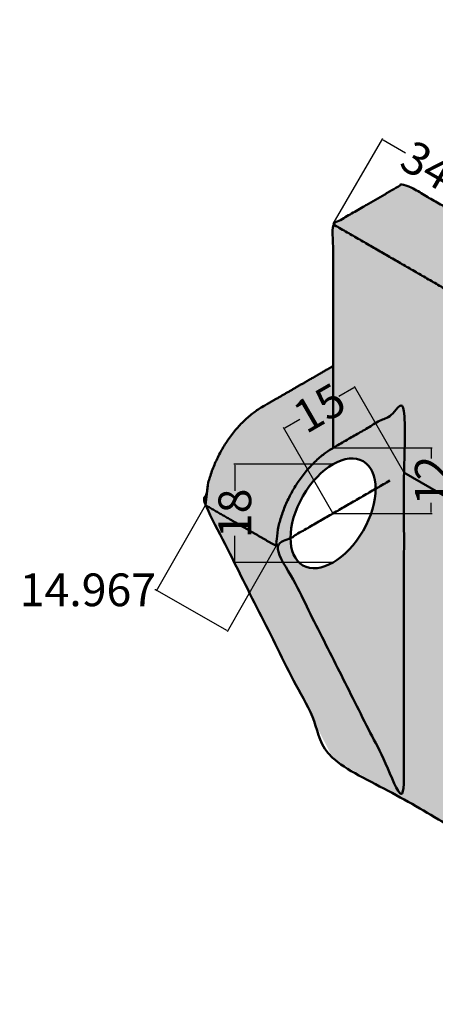
# Model space of a CAD drawing. Units: millimetres. Extents: x -57 to 165, y 2 to 198.
# Tile 1 of 1: x -57.4 to 18.8, y 17.5 to 198. Entities that reach past the tile are written whole.
import ezdxf

# ---------------------------------------------------------------- set-up
doc = ezdxf.new("R2010")
doc.units = ezdxf.units.MM
doc.header["$MEASUREMENT"] = 0
for name, color, linetype, lineweight in [('M-DIMS', 2, 'Continuous', 18), ('M-HATC', 8, 'Continuous', 18), ('M-OUTL', 7, 'Continuous', 50)]:
    doc.layers.add(name, color=color, linetype=linetype, lineweight=lineweight)
doc.styles.get("Standard").update_dxf_attribs({"font": 'arial.ttf'})
doc.dimstyles.get("Standard").update_dxf_attribs({"dimtxt": 6, "dimasz": 0.18, "dimexe": 0.18, "dimexo": 0.0625, "dimgap": 0.09, "dimtad": 0, "dimtoh": 1, "dimdec": 0, "dimzin": 0, "dimdsep": 46, "dimtxsty": 'Standard', "dimcen": 0.09, "dimadec": 0, "dimazin": 0, "dimtfac": 1, "dimtdec": 0, "dimtofl": 0, "dimtmove": 0, "dimatfit": 3, "dimfxl": 1, "dimtolj": 1, "dimtzin": 0, "dimarcsym": 0})

# ---------------------------------------------------------------- blocks, each defined once
blk = doc.blocks.new('*D13')
at = {"layer": 'Defpoints', "color": 0, "transparency": 16777216}
for p in [(-17.95371300000001, 116.497997), (0.046287, 116.497997), (0.046287, 98.49799700000005)]:
    blk.add_point(p, dxfattribs=at)
at = {"layer": 'M-DIMS', "color": 0, "lineweight": -2, "transparency": 16777216}
for p, q in [((-0.016213, 116.497997), (-18.13371300000001, 116.497997)), ((-17.95371300000001, 116.317997), (-17.95371300000001, 111.6091429754434)), ((-17.95371300000001, 98.67799700000006), (-17.95371300000001, 103.3868510245566)), ((-0.016213, 98.49799700000005), (-18.13371300000001, 98.49799700000005))]:
    blk.add_line(p, q, dxfattribs=at)
at = {"layer": 'M-DIMS', "color": 0, "transparency": 16777216}
for points in [[(-17.98371300000001, 116.317997), (-17.92371300000001, 116.317997), (-17.95371300000001, 116.497997)], [(-17.98371300000001, 98.67799700000006), (-17.92371300000001, 98.67799700000006), (-17.95371300000001, 98.49799700000005)]]:
    blk.add_solid(points, dxfattribs=at)
at = {"layer": 'M-DIMS', "color": 0, "transparency": 16777216, "insert": (-17.95371299999998, 107.497997), "char_height": 6, "attachment_point": 5, "rotation": 90}
blk.add_mtext('\\A1;18', dxfattribs=at)
blk = doc.blocks.new('*D17')
at = {"layer": 'Defpoints', "color": 0, "transparency": 16777216}
for p in [(0.0462869999999924, 160.497997), (39.30844832468702, 158.6118924312673), (30.307407, 143.024036)]:
    blk.add_point(p, dxfattribs=at)
at = {"layer": 'M-DIMS', "color": 0, "lineweight": -2, "transparency": 16777216}
for p, q in [((0.0775406150812756, 160.5521215004074), (9.137338633268897, 176.2417318143229)), ((9.203206783008142, 175.9958428417155), (13.32703206028853, 173.6145839495605)), ((39.1525697635137, 158.7019028427014), (35.0287444862333, 161.0831617348563)), ((30.33866061508128, 143.0781605004074), (39.39845873612112, 158.7677709924407))]:
    blk.add_line(p, q, dxfattribs=at)
at = {"layer": 'M-DIMS', "color": 0, "transparency": 16777216}
for points in [[(9.218208518247167, 176.021822601911), (9.18820504776913, 175.9698630815199), (9.047328221834803, 176.0858532531495)], [(39.16757149875272, 158.727882602897), (39.13756802827469, 158.6759230825059), (39.30844832468702, 158.6118924312673)]]:
    blk.add_solid(points, dxfattribs=at)
at = {"layer": 'M-DIMS', "color": 0, "transparency": 16777216, "insert": (24.17788827326091, 167.3488728422084), "char_height": 6, "attachment_point": 5, "rotation": 329.9961731765761}
blk.add_mtext('\\A1;34.944', dxfattribs=at)
blk = doc.blocks.new('*D19')
at = {"layer": 'Defpoints', "color": 0, "transparency": 16777216}
for p in [(0.046287, 119.497997), (0.046287, 107.497997), (18.04628700000001, 107.497997)]:
    blk.add_point(p, dxfattribs=at)
at = {"layer": 'M-DIMS', "color": 0, "lineweight": -2, "transparency": 16777216}
for p, q in [((0.108787, 119.497997), (18.22628700000001, 119.497997)), ((18.04628700000001, 119.317997), (18.04628700000001, 117.5723080504775)), ((18.04628700000001, 107.677997), (18.04628700000001, 109.4236859495225)), ((0.108787, 107.497997), (18.22628700000001, 107.497997))]:
    blk.add_line(p, q, dxfattribs=at)
at = {"layer": 'M-DIMS', "color": 0, "transparency": 16777216}
for points in [[(18.01628700000001, 119.317997), (18.07628700000001, 119.317997), (18.04628700000001, 119.497997)], [(18.01628700000001, 107.677997), (18.07628700000001, 107.677997), (18.04628700000001, 107.497997)]]:
    blk.add_solid(points, dxfattribs=at)
at = {"layer": 'M-DIMS', "color": 0, "transparency": 16777216, "insert": (18.04628700000004, 113.497997), "char_height": 6, "attachment_point": 5, "rotation": 90}
blk.add_mtext('\\A1;12', dxfattribs=at)
blk = doc.blocks.new('*D20')
at = {"layer": 'Defpoints', "color": 0, "transparency": 16777216}
for p in [(-23.334605, 109.012794), (-10.345802, 101.575348), (-32.2789480937495, 93.39233559130196)]:
    blk.add_point(p, dxfattribs=at)
at = {"layer": 'M-DIMS', "color": 0, "lineweight": -2, "transparency": 16777216}
for p, q in [((-23.36566174712761, 108.958556296713), (-32.368391525477, 93.2361310058353)), ((-10.3768587471276, 101.521110296713), (-19.37958837362152, 85.7986852710367)), ((-32.43515267921615, 93.48177902302945), (-32.61515267921615, 93.48177902302945)), ((-32.2789480937495, 93.39233559130196), (-32.43515267921615, 93.48177902302945)), ((-19.44634952736067, 86.04433328823085), (-32.12274350828284, 93.30289215957445))]:
    blk.add_line(p, q, dxfattribs=at)
at = {"layer": 'M-DIMS', "color": 0, "transparency": 16777216}
for points in [[(-32.1078362696616, 93.32892625715222), (-32.13765074690409, 93.27685806199668), (-32.2789480937495, 93.39233559130196)], [(-19.43144228873942, 86.07036738580862), (-19.46125676598192, 86.01829919065307), (-19.29014494189402, 85.95488985650334)]]:
    blk.add_solid(points, dxfattribs=at)
at = {"layer": 'M-DIMS', "color": 0, "transparency": 16777216, "insert": (-44.87704899572364, 93.48177902302946), "char_height": 6, "attachment_point": 5}
blk.add_mtext('\\A1;14.967', dxfattribs=at)
blk = doc.blocks.new('*D21')
at = {"layer": 'Defpoints', "color": 0, "transparency": 16777216}
for p in [(4.036668248195148, 130.5864538382333), (13.03666799999999, 114.997997), (0.0462869999999924, 107.497997)]:
    blk.add_point(p, dxfattribs=at)
at = {"layer": 'M-DIMS', "color": 0, "lineweight": -2, "transparency": 16777216}
for p, q in [((3.880783675513939, 130.4964538382333), (1.116012363729204, 128.9002123771266)), ((13.00541799999999, 115.0521235877365), (3.946668248195145, 130.7423384109145)), ((-8.797828193315297, 123.1764538628139), (-6.033056881530569, 124.7726953239206)), ((0.0150369999999924, 107.5521235877365), (-9.043712765996503, 123.2423384354951))]:
    blk.add_line(p, q, dxfattribs=at)
at = {"layer": 'M-DIMS', "color": 0, "transparency": 16777216}
for points in [[(3.865783675513938, 130.5224346003468), (3.895783675513939, 130.4704730761197), (4.036668248195148, 130.5864538382333)], [(-8.812828193315298, 123.2024346249275), (-8.782828193315297, 123.1504731007004), (-8.9537127659965, 123.0864538628139)]]:
    blk.add_solid(points, dxfattribs=at)
at = {"layer": 'M-DIMS', "color": 0, "transparency": 16777216, "insert": (-2.458522258900671, 126.8364538505236), "char_height": 6, "attachment_point": 5, "rotation": 29.999999999999993}
blk.add_mtext('\\A1;15', dxfattribs=at)

msp = doc.modelspace()

# ---------------------------------------------------------------- hatches: boundary and pattern name
at = {"layer": 'M-HATC'}
h = msp.add_hatch(color=256, dxfattribs=at)
h.set_gradient(color1=(16, 86, 137), color2=(147, 149, 152), tint=1)
h.paths.add_polyline_path([(95.30908161067455, 67.49799706451296), (125.6199707431299, 84.99799706451296), (125.6199707431299, 44.99799706451294), (142.9404788188187, 54.99799706451296), (142.9404788188187, 114.9979970645127), (77.98857353498579, 77.49799706451294), (77.98857353498579, 17.49799706451294), (95.30908161067455, 27.49799706451294)])
edge = h.paths.add_edge_path()
edge.add_spline(control_points=[(41.37988016936596, 131.3619580951918), (36.81412674377037, 139.2700750031551), (30.35717632684165, 142.9979970645129)], knot_values=[0, 0, 0, 0.7853981633974488, 0.7853981633974488, 0.7853981633974488], weights=[1, 0.9238795325112866, 1], degree=2, periodic=0)
edge.add_spline(control_points=[(30.35717632684165, 142.9979970645129), (15.20173176061398, 151.7479970645129), (0.0462871943863021, 160.4979970645129)], knot_values=[0.7853981633974488, 0.7853981633974488, 0.7853981633974488, 1.785398163397448, 1.785398163397448, 1.785398163397448], weights=[1, 1, 1], degree=2, periodic=0)
edge.add_spline(control_points=[(0.046287194386295, 160.4979970645129), (0.046287194386295, 147.4979970645129), (0.046287194386295, 134.4979970645129)], knot_values=[2.785398163397448, 2.785398163397448, 2.785398163397448, 3.419544504860864, 3.419544504860864, 3.419544504860864], weights=[1, 1, 1], degree=2, periodic=0)
edge.add_spline(control_points=[(0.046287194386295, 134.4979970645129), (0.046287194386295, 126.9979970645129), (0.046287194386295, 119.4979970645129)], knot_values=[3.419544504860864, 3.419544504860864, 3.419544504860864, 3.785398163397448, 3.785398163397448, 3.785398163397448], weights=[1, 1, 1], degree=2, periodic=0)
edge.add_spline(control_points=[(0.046287194386295, 119.4979970645129), (6.541477722769585, 123.2479970645129), (13.03666825115288, 126.9979970645129)], knot_values=[3, 3, 3, 4, 4, 4], weights=[1, 1, 1], degree=2, periodic=0)
edge.add_spline(control_points=[(13.03666825115288, 126.9979970645129), (13.03666825115288, 90.99799706451292), (13.03666825115288, 54.99799706451296)], knot_values=[2, 2, 2, 3, 3, 3], weights=[1, 1, 1], degree=2, periodic=0)
edge.add_line((13.03666825115287, 114.9979970645129), (77.98857353498579, 77.49799706451294))
edge.add_line((77.98857353498579, 77.49799706451294), (41.37988016936608, 131.3619580951916))
edge = h.paths.add_edge_path(flags=16)
edge.add_ellipse((30.35717632684166, 124.9979970645129), major_axis=(6.123724356957944, -10.60660171779821), ratio=0.577350269189626, start_angle=0, end_angle=360)
h.paths.add_polyline_path([(54.37026122613253, 138.8619580951918), (41.37988016936596, 131.3619580951918), (77.98857353498579, 77.49799706451294), (90.97895459175238, 84.99799706451292)])
edge = h.paths.add_edge_path()
edge.add_spline(control_points=[(45.75812342050349, 148.8897380148136), (44.56013330857391, 149.7979160278211), (43.34755738360823, 150.4979970645129)], knot_values=[0.6281854185381637, 0.6281854185381637, 0.6281854185381637, 0.7853981633974488, 0.7853981633974488, 0.7853981633974488], weights=[0.975625973363323, 0.9847630053244513, 1], degree=2, periodic=0)
edge.add_spline(control_points=[(43.34755738360823, 150.4979970645129), (28.19211281738056, 159.2479970645129), (13.03666825115287, 167.9979970645129)], knot_values=[0.7853981633974488, 0.7853981633974488, 0.7853981633974488, 1.785398163397448, 1.785398163397448, 1.785398163397448], weights=[1, 1, 1], degree=2, periodic=0)
edge.add_spline(control_points=[(13.03666825115287, 167.9979970645129), (6.541477722769585, 164.2479970645129), (0.046287194386295, 160.4979970645129)], knot_values=[1.785398163397448, 1.785398163397448, 1.785398163397448, 2.785398163397448, 2.785398163397448, 2.785398163397448], weights=[1, 1, 1], degree=2, periodic=0)
edge.add_spline(control_points=[(0.0462871943863021, 160.4979970645129), (15.20173176061398, 151.7479970645129), (30.35717632684165, 142.9979970645129)], knot_values=[0.7853981633974488, 0.7853981633974488, 0.7853981633974488, 1.785398163397448, 1.785398163397448, 1.785398163397448], weights=[1, 1, 1], degree=2, periodic=0)
edge.add_spline(control_points=[(30.35717632684165, 142.9979970645129), (36.81412674377037, 139.2700750031551), (41.37988016936596, 131.3619580951918)], knot_values=[0, 0, 0, 0.7853981633974488, 0.7853981633974488, 0.7853981633974488], weights=[1, 0.9238795325112866, 1], degree=2, periodic=0)
edge.add_line((41.37988016936598, 131.3619580951918), (54.37026122613254, 138.8619580951918))
edge.add_spline(control_points=[(54.37026122613254, 138.8619580951918), (50.7776825657607, 145.0844868651436), (45.75812342050349, 148.8897380148136)], knot_values=[0, 0, 0, 0.6281854185381637, 0.6281854185381637, 0.6281854185381637], weights=[1, 0.9391165271868352, 0.975625973363323], degree=2, periodic=0)
edge = h.paths.add_edge_path()
edge.add_spline(control_points=[(95.30908161067462, 180.4979970645128), (80.15363704444697, 189.2479970645128), (64.9981924782193, 197.9979970645128)], knot_values=[0.7853981633974488, 0.7853981633974488, 0.7853981633974488, 1.785398163397448, 1.785398163397448, 1.785398163397448], weights=[1, 1, 1], degree=2, periodic=0)
edge.add_spline(control_points=[(64.9981924782193, 197.9979970645128), (58.503001949836, 194.2479970645128), (52.0078114214527, 190.4979970645127)], knot_values=[1.785398163397448, 1.785398163397448, 1.785398163397448, 2.785398163397447, 2.785398163397448, 2.785398163397448], weights=[1, 1, 1], degree=2, periodic=0)
edge.add_spline(control_points=[(52.00781142145273, 190.4979970645127), (67.1632559876804, 181.7479970645128), (82.31870055390804, 172.9979970645128)], knot_values=[0.7853981633974488, 0.7853981633974488, 0.7853981633974488, 1.785398163397448, 1.785398163397448, 1.785398163397448], weights=[1, 1, 1], degree=2, periodic=0)
edge.add_spline(control_points=[(82.31870055390804, 172.9979970645128), (88.77565097083676, 169.2700750031549), (93.34140439643235, 161.3619580951917)], knot_values=[0, 0, 0, 0.7853981633974488, 0.7853981633974488, 0.7853981633974488], weights=[1, 0.9238795325112866, 1], degree=2, periodic=0)
edge.add_line((93.34140439643235, 161.3619580951917), (106.3317854531989, 168.8619580951917))
edge.add_spline(control_points=[(106.3317854531989, 168.8619580951917), (101.7660320276033, 176.7700750031549), (95.30908161067462, 180.4979970645128)], knot_values=[0, 0, 0, 0.7853981633974488, 0.7853981633974488, 0.7853981633974488], weights=[1, 0.9238795325112866, 1], degree=2, periodic=0)
h.paths.add_polyline_path([(106.3317854531989, 168.8619580951917), (93.34140439643235, 161.3619580951917), (129.9500977620521, 107.4979970645128), (142.9404788188187, 114.9979970645128)])
edge = h.paths.add_edge_path()
edge.add_spline(control_points=[(93.34140439643235, 161.3619580951917), (88.77565097083676, 169.2700750031549), (82.31870055390804, 172.9979970645128)], knot_values=[0, 0, 0, 0.7853981633974488, 0.7853981633974488, 0.7853981633974488], weights=[1, 0.9238795325112866, 1], degree=2, periodic=0)
edge.add_spline(control_points=[(82.31870055390804, 172.9979970645128), (67.1632559876804, 181.7479970645128), (52.00781142145273, 190.4979970645127)], knot_values=[0.7853981633974488, 0.7853981633974488, 0.7853981633974488, 1.785398163397448, 1.785398163397448, 1.785398163397448], weights=[1, 1, 1], degree=2, periodic=0)
edge.add_spline(control_points=[(52.0078114214527, 190.4979970645127), (52.0078114214527, 171.4979970645128), (52.0078114214527, 152.4979970645128)], knot_values=[2.785398163397447, 2.785398163397448, 2.785398163397448, 3.785398163397448, 3.785398163397448, 3.785398163397448], weights=[1, 1, 1], degree=2, periodic=0)
edge.add_line((52.0078114214527, 152.4979970645128), (129.9500977620521, 107.4979970645128))
edge.add_line((129.9500977620521, 107.4979970645128), (93.34140439643232, 161.3619580951917))
edge = h.paths.add_edge_path(flags=16)
edge.add_ellipse((82.31870055390804, 154.9979970645128), major_axis=(6.123724356957944, -10.60660171779821), ratio=0.577350269189626, start_angle=0, end_angle=360)
edge = h.paths.add_edge_path()
edge.add_line((52.0078114214527, 152.4979970645128), (45.7581234205035, 148.8897380148136))
edge.add_spline(control_points=[(45.75812342050349, 148.8897380148136), (50.7776825657607, 145.0844868651436), (54.37026122613254, 138.8619580951918)], knot_values=[0, 0, 0, 0.6281854185381637, 0.6281854185381637, 0.6281854185381637], weights=[0.975625973363323, 0.9391165271868352, 1], degree=2, periodic=0)
edge.add_line((54.37026122613257, 138.8619580951917), (75.66970573764932, 107.5231600210469))
edge.add_ellipse((90.97895459175238, 107.4979970645129), major_axis=(-15.30931089239486, 0), ratio=0.577350269189626, start_angle=330, end_angle=359.90582621493047, ccw=False)
edge.add_line((80.1536370444469, 113.7479970645129), (71.49338300660253, 118.7479970645128))
edge.add_line((71.49338300660253, 118.7479970645128), (90.97895459175236, 129.9979970645128))
edge.add_line((90.97895459175236, 129.9979970645128), (52.0078114214527, 152.4979970645128))
edge = h.paths.add_edge_path()
edge.add_line((90.97895459175236, 129.9979970645128), (71.49338300660254, 118.7479970645128))
edge.add_line((71.49338300660254, 118.7479970645128), (80.15363704444688, 113.7479970645129))
edge.add_ellipse((90.97895459175238, 107.4979970645129), major_axis=(-15.30931089239486, 0), ratio=0.577350269189626, start_angle=150.0000000000001, end_angle=330, ccw=False)
edge.add_line((101.8042721390579, 101.2479970645129), (110.4645261769023, 96.24799706451292))
edge.add_line((110.4645261769023, 96.24799706451292), (129.9500977620521, 107.4979970645128))
edge.add_line((129.9500977620521, 107.4979970645128), (90.97895459175236, 129.9979970645128))
edge = h.paths.add_edge_path(flags=17)
edge.add_line((110.4645261769023, 96.24799706451292), (101.8042721390579, 101.2479970645129))
edge.add_ellipse((90.97895459175238, 107.4979970645129), major_axis=(-15.30931089239486, 0), ratio=0.577350269189626, start_angle=28.308251316207816, end_angle=150.0000000000001, ccw=False)
edge.add_line((79.784778540041, 101.4684746256213), (90.97895459175238, 84.99799706451292))
edge.add_line((90.97895459175238, 84.99799706451292), (110.4645261769023, 96.24799706451292))
edge = h.paths.add_edge_path()
edge.add_line((77.98857353498579, 77.49799706451294), (13.03666825115287, 114.9979970645129))
edge.add_spline(control_points=[(13.03666825115288, 114.9979970645129), (13.03666825115288, 84.99799706451293), (13.03666825115288, 54.99799706451296)], knot_values=[2, 2, 2, 2.833333333333333, 2.833333333333333, 2.833333333333333], weights=[1, 1, 1], degree=2, periodic=0)
edge.add_spline(control_points=[(13.03666825115288, 54.99799706451296), (45.51262089306933, 36.24799706451295), (77.98857353498579, 17.49799706451294)], knot_values=[3.737462993461563, 3.737462993461563, 3.737462993461563, 4.570796326794897, 4.570796326794897, 4.570796326794897], weights=[1, 1, 1], degree=2, periodic=0)
edge.add_line((77.98857353498579, 17.49799706451294), (77.98857353498579, 77.49799706451294))
edge = h.paths.add_edge_path()
edge.add_spline(control_points=[(13.03666825115288, 54.99799706451296), (13.03666825115288, 84.99799706451293), (13.03666825115288, 114.9979970645129)], knot_values=[2, 2, 2, 2.833333333333333, 2.833333333333333, 2.833333333333333], weights=[1, 1, 1], degree=2, periodic=0)
edge.add_spline(control_points=[(13.03666825115288, 114.9979970645129), (13.03666825115288, 120.9979970645129), (13.03666825115288, 126.9979970645129)], knot_values=[2.833333333333333, 2.833333333333333, 2.833333333333333, 3, 3, 3], weights=[1, 1, 1], degree=2, periodic=0)
edge.add_spline(control_points=[(13.03666825115288, 126.9979970645129), (6.541477722769585, 123.2479970645129), (0.046287194386295, 119.4979970645129)], knot_values=[3, 3, 3, 4, 4, 4], weights=[1, 1, 1], degree=2, periodic=0)
edge.add_spline(control_points=[(0.046287194386295, 119.4979970645129), (-4.258346416899511, 117.0127156902743), (-7.302182033963242, 111.7406377516322), (-10.34601765102697, 106.46855981299), (-10.34601765102697, 101.4979970645129)], knot_values=[4, 4, 4, 4.785398163397448, 4.785398163397448, 5.570796326794897, 5.570796326794897, 5.570796326794897], weights=[1, 0.9238795325112866, 1, 0.9238795325112866, 1], degree=2, periodic=0)
edge.add_spline(control_points=[(-10.34601765102697, 101.4979970645129), (-9.046979545350315, 102.2479970645129), (-7.747941439673653, 102.9979970645129)], knot_values=[0.8749999999999998, 0.8749999999999998, 0.8749999999999998, 1, 1, 1], weights=[1, 1, 1], degree=2, periodic=0)
edge.add_ellipse((0.0462871943862933, 107.4979970645129), major_axis=(-5.511351921262146, -9.545941546018396), ratio=0.577350269189626, start_angle=150, end_angle=330, ccw=False)
edge.add_ellipse((0.0462871943862933, 107.4979970645129), major_axis=(-5.511351921262146, -9.545941546018396), ratio=0.577350269189626, start_angle=330, end_angle=509.9999999999999, ccw=False)
edge.add_spline(control_points=[(-7.747941439673653, 102.9979970645129), (-9.046979545350315, 102.2479970645129), (-10.34601765102697, 101.4979970645129)], knot_values=[0.8749999999999998, 0.8749999999999998, 0.8749999999999998, 1, 1, 1], weights=[1, 1, 1], degree=2, periodic=0)
edge.add_spline(control_points=[(-10.34601765102697, 101.4979970645129), (1.345325300062951, 78.24799706451296), (13.03666825115288, 54.99799706451296)], knot_values=[1, 1, 1, 2, 2, 2], weights=[1, 1, 1], degree=2, periodic=0)
edge = h.paths.add_edge_path()
edge.add_spline(control_points=[(0.046287194386295, 119.4979970645129), (0.046287194386295, 126.9979970645129), (0.046287194386295, 134.4979970645129)], knot_values=[3.419544504860864, 3.419544504860864, 3.419544504860864, 3.785398163397449, 3.785398163397449, 3.785398163397449], weights=[1, 1, 1], degree=2, periodic=0)
edge.add_spline(control_points=[(0.0462871943863093, 134.4979970645129), (-6.448903333996982, 130.7479970645129), (-12.94409386238027, 126.9979970645129)], knot_values=[0, 0, 0, 1, 1, 1], weights=[1, 1, 1], degree=2, periodic=0)
edge.add_spline(control_points=[(-12.94409386238027, 126.9979970645129), (-17.24872747366608, 124.5127156902743), (-20.29256309072981, 119.2406377516322), (-22.11694969149519, 116.0807074664587), (-22.87621616226442, 112.7950566133887)], knot_values=[1, 1, 1, 1.785398163397448, 1.785398163397448, 2.27095043198655, 2.27095043198655, 2.27095043198655], weights=[1, 0.9238795325112866, 1, 0.9529404735104989, 0.9640676373154162], degree=2, periodic=0)
edge.add_spline(control_points=[(-22.87621616226443, 112.7950566133887), (-23.10630743502899, 110.8965268389508), (-23.33639870779354, 108.9979970645129)], knot_values=[6.570796326794897, 6.570796326794897, 6.570796326794897, 7.570796326794897, 7.570796326794897, 7.570796326794897], weights=[1, 1, 1], degree=2, periodic=0)
edge.add_spline(control_points=[(-23.33639870779354, 108.9979970645129), (-16.84120817941026, 105.2479970645129), (-10.34601765102697, 101.4979970645129)], knot_values=[5.570796326794897, 5.570796326794897, 5.570796326794897, 6.570796326794897, 6.570796326794897, 6.570796326794897], weights=[1, 1, 1], degree=2, periodic=0)
edge.add_spline(control_points=[(-10.34601765102697, 101.4979970645129), (-10.34601765102697, 106.46855981299), (-7.302182033963242, 111.7406377516322), (-4.258346416899511, 117.0127156902743), (0.046287194386295, 119.4979970645129)], knot_values=[4, 4, 4, 4.78539816339745, 4.78539816339745, 5.570796326794898, 5.570796326794898, 5.570796326794898], weights=[1, 0.9238795325112866, 1, 0.9238795325112866, 1], degree=2, periodic=0)
edge = h.paths.add_edge_path()
edge.add_spline(control_points=[(-10.34601765102697, 101.4979970645129), (-16.84120817941026, 105.2479970645129), (-23.33639870779354, 108.9979970645129)], knot_values=[5.570796326794897, 5.570796326794897, 5.570796326794897, 6.570796326794897, 6.570796326794897, 6.570796326794897], weights=[1, 1, 1], degree=2, periodic=0)
edge.add_spline(control_points=[(-23.33639870779354, 108.9979970645129), (-11.64505575670361, 85.74799706451296), (0.0462871943863093, 62.49799706451296)], knot_values=[2.570796326772039, 2.570796326794897, 2.570796326794897, 3.570796326794897, 3.570796326794897, 3.570796326794897], weights=[1, 1, 1], degree=2, periodic=0)
edge.add_spline(control_points=[(0.0462871943863093, 62.49799706451296), (6.541477722769593, 58.74799706451296), (13.03666825115288, 54.99799706451296)], knot_values=[3.570796326794897, 3.570796326794897, 3.570796326794897, 3.737462993461563, 3.737462993461563, 3.737462993461563], weights=[1, 1, 1], degree=2, periodic=0)
edge.add_spline(control_points=[(13.03666825115288, 54.99799706451296), (1.345325300062951, 78.24799706451296), (-10.34601765102697, 101.4979970645129)], knot_values=[1, 1, 1, 2, 2, 2], weights=[1, 1, 1], degree=2, periodic=0)

# ---------------------------------------------------------------- linework, layer by layer
at = {"layer": 'M-OUTL'}
msp.add_lwpolyline([(13.03666825115288, 114.9979970645129), (77.98857353498579, 77.49799706451294), (41.37988016936597, 131.3619580951918), (54.37026122613253, 138.8619580951918), (90.97895459175237, 84.99799706451294)], dxfattribs=at)
msp.add_ellipse((0.0462871943862933, 107.4979970645129), major_axis=(-5.511351921262144, -9.545941546018392), ratio=0.5773502691896258, dxfattribs=at)
for points, weights, knots in [([(54.37026122613254, 138.8619580951918), (49.80450780053694, 146.7700750031551), (43.34755738360823, 150.4979970645129), (28.19211281738056, 159.2479970645129), (13.03666825115287, 167.9979970645129), (6.541477722769585, 164.2479970645129), (0.046287194386295, 160.4979970645129), (0.046287194386295, 139.9979970645129), (0.046287194386295, 119.4979970645129)], [1, 0.9238795325112866, 1, 1, 1, 1, 1, 1, 1], [0, 0, 0, 0.7853981633974488, 0.7853981633974488, 1.785398163397448, 1.785398163397448, 2.785398163397448, 2.785398163397448, 3.785398163397448, 3.785398163397448, 3.785398163397448]), ([(41.37988016936596, 131.3619580951918), (36.81412674377037, 139.2700750031551), (30.35717632684165, 142.9979970645129), (15.20173176061398, 151.7479970645129), (0.0462871943863021, 160.4979970645129)], [1, 0.9238795325112866, 1, 1, 1], [0, 0, 0, 0.7853981633974488, 0.7853981633974488, 1.785398163397448, 1.785398163397448, 1.785398163397448]), ([(0.0462871943863093, 134.4979970645129), (-6.448903333996982, 130.7479970645129), (-12.94409386238027, 126.9979970645129), (-17.24872747366608, 124.5127156902743), (-20.29256309072981, 119.2406377516322), (-23.33639870779354, 113.9685598129901), (-23.33639870779354, 108.9979970645129), (-11.64505575670361, 85.74799706451296), (0.0462871943863093, 62.49799706451296), (39.01743036468605, 39.99799706451295), (77.98857353498579, 17.49799706451294)], [1, 1, 1, 0.9238795325112866, 1, 0.9238795325112866, 1, 1, 1, 1, 1], [0, 0, 0, 1, 1, 1.785398163397448, 1.785398163397448, 2.570796326794897, 2.570796326794897, 3.570796326794897, 3.570796326794897, 4.570796326794897, 4.570796326794897, 4.570796326794897]), ([(10.43859203979956, 113.4979970645129), (0.0462871943862933, 107.4979970645129), (-10.34601765102697, 101.4979970645129), (1.345325300062951, 78.24799706451296), (13.03666825115288, 54.99799706451296), (13.03666825115288, 90.99799706451292), (13.03666825115288, 126.9979970645129), (6.541477722769585, 123.2479970645129), (0.046287194386295, 119.4979970645129), (-4.258346416899511, 117.0127156902743), (-7.302182033963242, 111.7406377516322), (-10.34601765102697, 106.46855981299), (-10.34601765102697, 101.4979970645129), (-16.84120817941026, 105.2479970645129), (-23.33639870779354, 108.9979970645129), (-23.10630743502899, 110.8965268389508), (-22.87621616226443, 112.7950566133887)], [1, 1, 1, 1, 1, 1, 1, 1, 1, 0.9238795325112866, 1, 0.9238795325112866, 1, 1, 1, 1, 1], [0, 0, 0, 1, 1, 2, 2, 3, 3, 4, 4, 4.785398163397448, 4.785398163397448, 5.570796326794897, 5.570796326794897, 6.570796326794897, 6.570796326794897, 7.570796326794897, 7.570796326794897, 7.570796326794897])]:
    msp.add_rational_spline(points, weights, degree=2, knots=knots, dxfattribs=at)

# ---------------------------------------------------------------- dimensions: what is measured, and where the dimension line sits
at = {"layer": 'M-DIMS'}
for base, p1, p2, angle, override, picture, middle in [((39.30844832468702, 158.6118924312673), (0.046287, 160.497997), (30.307407, 143.024036), 329.9961731765761, {"dimdec": 3, "dimlfac": 1, "dimrnd": 0, "dimzin": 0, "dimdsep": 46, "dimlunit": 2}, '*D17', (24.17788827326091, 167.3488728422084)), ((4.036668248195148, 130.5864538382333), (0.046287, 107.497997), (13.036668, 114.997997), 29.99999999999999, {"dimdec": 0, "dimlfac": 1, "dimrnd": 0, "dimzin": 0, "dimdsep": 46, "dimlunit": 2}, '*D21', (-2.458522258900671, 126.8364538505236)), ((18.04628700000001, 107.497997), (0.046287, 119.497997), (0.046287, 107.497997), 270, {"dimdec": 0, "dimlfac": 1, "dimrnd": 0, "dimzin": 0, "dimdsep": 46, "dimlunit": 2}, '*D19', (18.04628700000004, 113.497997)), ((-17.95371300000001, 116.497997), (0.046287, 98.497997), (0.046287, 116.497997), 90.00000000000003, {"dimdec": 0, "dimlfac": 1, "dimrnd": 0, "dimzin": 0, "dimdsep": 46, "dimlunit": 2}, '*D13', (-17.95371299999998, 107.497997)), ((-32.2789480937495, 93.39233559130196), (-10.345802, 101.575348), (-23.334605, 109.012794), 150.2043581353996, {"dimdec": 3, "dimlfac": 1, "dimrnd": 0, "dimzin": 0, "dimdsep": 46, "dimlunit": 2}, '*D20', (-44.87704899572364, 93.48177902302946))]:
    dim = msp.add_linear_dim(base=base, p1=p1, p2=p2, angle=angle, dimstyle='Standard', override=override, dxfattribs=at)
    dim.commit()
    dim.dimension.update_dxf_attribs({"geometry": picture, "text_midpoint": middle})

doc.saveas('drawing.dxf')
